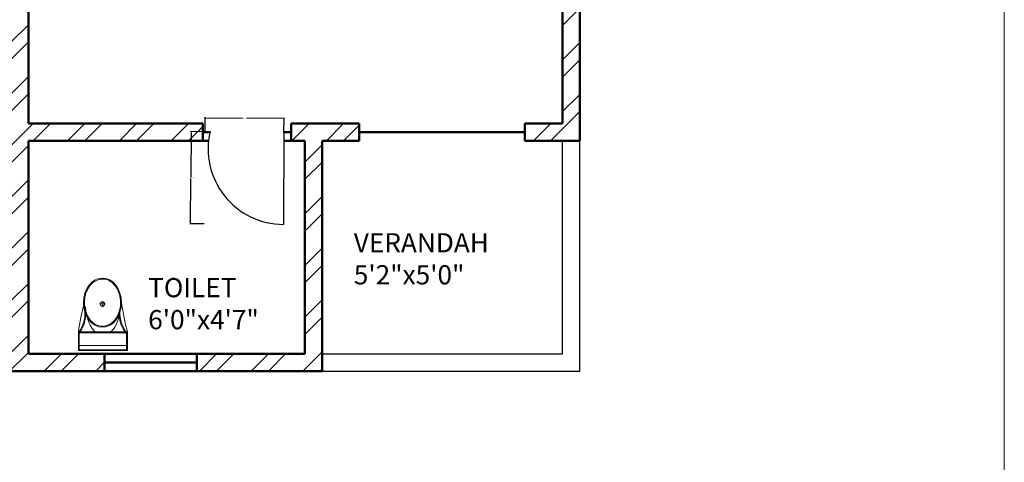
# Model space of a CAD drawing. Units: inches. Extents: x 1901 to 2863, y 888 to 2433.
# Tile 33 of 91: x 2607 to 2863, y 1175 to 1291. Entities that reach past the tile are written whole.
import ezdxf

# ---------------------------------------------------------------- set-up
doc = ezdxf.new("R2010")
doc.units = ezdxf.units.IN
for name, color, linetype, lineweight in [('A-ANNO-DIMS', 2, 'Continuous', 18), ('A-AREA-IDEN', 7, 'Continuous', 18), ('A-DOOR', 4, 'Continuous', 25), ('A-FLOR-FIXT', 9, 'Continuous', 18), ('A-FLOR-HRAL', 41, 'Continuous', 25), ('A-WALL', 7, 'Continuous', 50), ('A-WALL-PATT', 8, 'Continuous', 13)]:
    doc.layers.add(name, color=color, linetype=linetype, lineweight=lineweight)
doc.styles.get("Standard").update_dxf_attribs({"font": 'arial.ttf'})
doc.dimstyles.get("Standard").update_dxf_attribs({"dimtxt": 0.18, "dimasz": 0.18, "dimexe": 0.18, "dimexo": 0.0625, "dimgap": 0.09, "dimtad": 0, "dimtih": 1, "dimtoh": 1, "dimdec": 4, "dimzin": 0, "dimdsep": 46, "dimtxsty": 'Standard', "dimcen": 0.09, "dimadec": 0, "dimazin": 0, "dimtfac": 1, "dimtdec": 4, "dimtofl": 0, "dimtmove": 0, "dimatfit": 3, "dimfxl": 1, "dimtolj": 1, "dimtzin": 0, "dimarcsym": 0})

# ---------------------------------------------------------------- blocks, each defined once
blk = doc.blocks.new('A$C31115884')
for p, q in [((258, 466), (258, 523)), ((283, 498), (223, 498)), ((0, 200), (0, 0)), ((520, 200), (0, 200)), ((10, 190), (10, 10)), ((510, 190), (10, 190)), ((510, 10), (510, 190)), ((520, 0), (520, 200)), ((510, 54), (0, 54)), ((10, 10), (510, 10)), ((0, 0), (520, 0))]:
    blk.add_line(p, q)
blk.add_circle((256, 496), 23.6)
for centre, radius, start, end in [((2778, -205), 2807, 165.4549, 171.7133), ((-295, 403), 365, 324.2091, 9.3499), ((-295, 403), 375, 324.2091, 9.3499), ((139, 406), 293, 315.8436, 2.6563), ((806, 403), 365, 170.6501, 215.7909), ((3237, 905), 2807, 188.2867, 194.5451), ((384, 406), 293, 190.2774, 224.1564), ((806, 403), 375, 179.2036, 215.7909)]:
    blk.add_arc(centre, radius, start, end)
blk.add_ellipse((256, 510), major_axis=(0, -261), ratio=0.772727)
blk.add_open_spline([(256, 259), (263, 259), (270, 260), (288, 262), (299, 265), (320, 273), (330, 278), (350, 291), (360, 299), (378, 316), (386, 326), (402, 347), (409, 358), (421, 383), (427, 395), (436, 422), (440, 436), (445, 465), (447, 480), (448, 509), (448, 524), (445, 553), (443, 568), (436, 596), (432, 610), (422, 636), (416, 649), (402, 672), (395, 683), (379, 703), (370, 712), (351, 728), (341, 735), (321, 746), (310, 751), (289, 757), (278, 759), (256, 761), (245, 761), (223, 757), (212, 754), (191, 746), (181, 741), (161, 728), (151, 720), (133, 703), (125, 693), (110, 672), (103, 660), (90, 636), (85, 623), (76, 596), (72, 582), (67, 553), (66, 538), (64, 509), (65, 494), (68, 465), (70, 450), (77, 422), (81, 408), (91, 382), (97, 370), (111, 346), (118, 335), (135, 316), (144, 307), (162, 291), (172, 284), (193, 273), (203, 269), (225, 262), (236, 260), (250, 259), (253, 259), (256, 259)], degree=3, knots=[0, 0, 0, 0, 0.110105, 0.110105, 0.285049, 0.285049, 0.459994, 0.459994, 0.634938, 0.634938, 0.809882, 0.809882, 0.984827, 0.984827, 1.159771, 1.159771, 1.334715, 1.334715, 1.50966, 1.50966, 1.684604, 1.684604, 1.859549, 1.859549, 2.034493, 2.034493, 2.209437, 2.209437, 2.384382, 2.384382, 2.559326, 2.559326, 2.73427, 2.73427, 2.909215, 2.909215, 3.084159, 3.084159, 3.259103, 3.259103, 3.434048, 3.434048, 3.608992, 3.608992, 3.783936, 3.783936, 3.958881, 3.958881, 4.133825, 4.133825, 4.30877, 4.30877, 4.483714, 4.483714, 4.658658, 4.658658, 4.833603, 4.833603, 5.008547, 5.008547, 5.183491, 5.183491, 5.358436, 5.358436, 5.53338, 5.53338, 5.708324, 5.708324, 5.883269, 5.883269, 6.058213, 6.058213, 6.233158, 6.233158, 6.283185, 6.283185, 6.283185, 6.283185])
blk = doc.blocks.new('DOOR-20')
blk.add_line((0, -0.02), (0, 23.98))
blk.add_arc((0, 4.28), 19.71, 347.419, 90)
blk = doc.blocks.new('*D37')
at = {"layer": 'A-ANNO-DIMS', "color": 0, "lineweight": -2, "transparency": 16777216}
for p, q in [((2655.34, 1261.46), (2651.63, 1261.48)), ((2651.81, 1261.3), (2651.73, 1249.66)), ((2651.66, 1237.66), (2651.73, 1249.3)), ((2655.19, 1237.46), (2651.48, 1237.48))]:
    blk.add_line(p, q, dxfattribs=at)
at = {"layer": 'A-ANNO-DIMS', "color": 0, "transparency": 16777216}
for points in [[(2651.78, 1261.3), (2651.84, 1261.3), (2651.81, 1261.48)], [(2651.63, 1237.66), (2651.69, 1237.66), (2651.66, 1237.48)]]:
    blk.add_solid(points, dxfattribs=at)
at = {"layer": 'Defpoints', "color": 0, "transparency": 16777216}
for p in [(2655.41, 1261.46), (2651.66, 1237.48), (2655.26, 1237.46)]:
    blk.add_point(p, dxfattribs=at)
at = {"layer": 'A-ANNO-DIMS', "color": 0, "transparency": 16777216, "insert": (2651.73, 1249.48), "char_height": 0.18, "attachment_point": 5}
blk.add_mtext('\\A1;DOOR D4 24 TYP.', dxfattribs=at)
blk = doc.blocks.new('*D38')
at = {"layer": 'A-ANNO-DIMS', "color": 0, "lineweight": -2, "transparency": 16777216}
for p, q in [((2655.41, 1261.52), (2655.43, 1265.24)), ((2655.61, 1265.06), (2665.17, 1265)), ((2675.79, 1264.93), (2666.23, 1264.99)), ((2675.94, 1261.39), (2675.97, 1265.11))]:
    blk.add_line(p, q, dxfattribs=at)
at = {"layer": 'A-ANNO-DIMS', "color": 0, "transparency": 16777216}
for points in [[(2655.61, 1265.09), (2655.61, 1265.03), (2655.43, 1265.06)], [(2675.79, 1264.96), (2675.79, 1264.9), (2675.97, 1264.93)]]:
    blk.add_solid(points, dxfattribs=at)
at = {"layer": 'Defpoints', "color": 0, "transparency": 16777216}
for p in [(2655.43, 1265.06), (2655.41, 1261.46), (2675.94, 1261.33)]:
    blk.add_point(p, dxfattribs=at)
at = {"layer": 'A-ANNO-DIMS', "color": 0, "transparency": 16777216, "insert": (2665.7, 1264.99), "char_height": 0.18, "attachment_point": 5}
blk.add_mtext('\\A1;21 TYP.', dxfattribs=at)

msp = doc.modelspace()

# ---------------------------------------------------------------- hatches: boundary and pattern name
at = {"layer": 'A-WALL-PATT'}
h = msp.add_hatch(dxfattribs=at)
h.set_pattern_fill('ANSI32', color=256)
h.paths.add_polyline_path([(2192.5, 2274.13), (2141.26, 2274.13), (2141.26, 2269.63), (2192.5, 2269.63)])
h.paths.add_polyline_path([(2259.93, 2274.13), (2216.5, 2274.13), (2216.5, 2269.63), (2255.43, 2269.63), (2255.43, 2214.63), (2250.81, 2214.63), (2250.81, 2210.13), (2259.93, 2210.13), (2259.93, 2215.13), (2271.76, 2215.13), (2271.76, 2217.38), (2271.76, 2219.63), (2259.93, 2219.63)])
h.paths.add_polyline_path([(2171.43, 2269.63), (2166.93, 2269.63), (2166.93, 2219.63), (2121.24, 2219.63), (2121.24, 2215.13), (2166.93, 2215.13), (2166.93, 2083.13), (2161.81, 2083.13), (2161.81, 2078.63), (2171.43, 2078.63), (2177, 2078.63), (2177, 2080.88), (2177, 2083.13), (2171.43, 2083.13), (2171.43, 2210.13), (2230.91, 2210.13), (2230.91, 2212.38), (2230.91, 2214.63), (2171.43, 2214.63)])
h.paths.add_polyline_path([(2117.26, 2274.13), (2089.43, 2274.13), (2089.43, 2219.63), (2081.14, 2219.63), (2081.14, 2215.13), (2089.43, 2215.13), (2098, 2215.13), (2098, 2217.38), (2098, 2219.63), (2093.93, 2219.63), (2093.93, 2269.63), (2117.26, 2269.63), (2117.26, 2271.88)])
h.paths.add_polyline_path([(2343.43, 2219.63), (2329.29, 2219.63), (2329.29, 2215.13), (2338.93, 2215.13), (2338.93, 2184.74), (2343.43, 2184.74)])
h.paths.add_polyline_path([(2338.93, 2083.13), (2329.29, 2083.13), (2208.97, 2083.13), (2208.97, 2078.63), (2338.93, 2078.63)])
h.paths.add_polyline_path([(2343.43, 2136.74), (2338.93, 2136.74), (2338.93, 1872.63), (2343.43, 1872.63)])
h.paths.add_polyline_path([(2343.43, 1863.63), (2397.68, 1863.63), (2397.68, 1821.63), (2384.14, 1821.63), (2384.14, 1812.63), (2418.33, 1812.63), (2418.33, 1817.13), (2418.33, 1821.63), (2406.68, 1821.63), (2406.68, 1863.63), (2459.5, 1863.63), (2459.5, 1821.63), (2447.14, 1821.63), (2447.14, 1812.63), (2459.5, 1812.63), (2468.5, 1812.63), (2468.5, 1872.63), (2394.43, 1872.63), (2334.43, 1872.63), (2334.43, 1812.63), (2343.43, 1812.63), (2353.25, 1812.63), (2353.25, 1821.63), (2343.43, 1821.63)])
h.paths.add_polyline_path([(2510.01, 1872.63), (2468.5, 1872.63), (2468.5, 1868.13), (2510.01, 1868.13)])
h.paths.add_polyline_path([(2514.01, 1817.13), (2468.5, 1817.13), (2468.5, 1812.63), (2482.11, 1812.63), (2482.11, 1800.61), (2486.61, 1800.61), (2486.61, 1812.63), (2514.01, 1812.63)])
h.paths.add_polyline_path([(2299.25, 1814.88), (2299.25, 1817.13), (2295.93, 1817.13), (2295.93, 1854.17), (2293.68, 1854.17), (2291.43, 1854.17), (2291.43, 1817.13), (2266.11, 1817.13), (2266.11, 1812.63), (2299.25, 1812.63)])
h.paths.add_polyline_path([(2218.11, 1817.13), (2206.46, 1817.13), (2171.43, 1817.13), (2171.43, 1949.13), (2190.1, 1949.13), (2190.1, 1953.63), (2163.47, 1953.63), (2163.47, 1949.13), (2166.93, 1949.13), (2166.93, 1817.13), (2114.3, 1817.13), (2114.3, 1812.63), (2218.11, 1812.63)])
h.paths.add_polyline_path([(2029.43, 1970.92), (2024.93, 1970.92), (2024.93, 1912.72), (2029.43, 1912.72)])
h.paths.add_polyline_path([(2132.3, 1953.63), (2113.93, 1953.63), (2113.93, 1975.89), (2111.68, 1975.89), (2109.43, 1975.89), (2109.43, 1953.63), (2029.43, 1953.63), (2029.43, 1949.13), (2132.3, 1949.13)])
h.paths.add_polyline_path([(2029.43, 1853.61), (2029.31, 1853.61), (2029.31, 1853.61), (2029.43, 1853.61), (2029.43, 1864.72), (2024.93, 1864.72), (2024.93, 1812.63), (2066.3, 1812.63), (2066.3, 1814.88), (2066.3, 1817.13), (2029.43, 1817.13)])
h.paths.add_polyline_path([(2122.93, 2010.09), (2120.68, 2010.09), (2118.43, 2010.09), (2118.43, 2006.13), (2029.43, 2006.13), (2029.43, 2001.63), (2109.43, 2001.63), (2109.43, 1998.04), (2113.93, 1998.04), (2113.93, 2001.63), (2122.93, 2001.63)])
h.paths.add_polyline_path([(2029.43, 2031.38), (2024.93, 2031.38), (2024.93, 1994.92), (2027.18, 1994.92), (2029.43, 1994.92)])
h.paths.add_polyline_path([(2029.43, 2136.74), (2024.93, 2136.74), (2024.93, 2067.38), (2027.18, 2067.38), (2029.43, 2067.38)])
h.paths.add_polyline_path([(2125.62, 2083.13), (2029.43, 2083.13), (2029.43, 2078.63), (2118.43, 2078.63), (2118.43, 2030.71), (2122.93, 2030.71), (2122.93, 2078.63), (2125.62, 2078.63)])
h.paths.add_polyline_path([(2029.43, 2215.13), (2040.47, 2215.13), (2040.47, 2217.38), (2040.47, 2219.63), (2024.93, 2219.63), (2024.93, 2184.74), (2029.43, 2184.74), (2029.43, 2187.78)])
h.paths.add_polyline_path([(2686.43, 2274.13), (2659.28, 2274.13), (2659.28, 2269.63), (2681.93, 2269.63), (2681.93, 2219.63), (2676.82, 2219.63), (2676.82, 2215.13), (2681.93, 2215.13), (2697.01, 2215.13), (2697.01, 2217.38), (2697.01, 2219.63), (2686.43, 2219.63)])
h.paths.add_polyline_path([(2609.93, 2269.63), (2635.28, 2269.63), (2635.28, 2274.13), (2571.43, 2274.13), (2571.43, 2269.63), (2605.43, 2269.63), (2605.43, 2214.63), (2549.1, 2214.63), (2549.1, 2210.13), (2605.43, 2210.13), (2605.43, 2083.13), (2601.01, 2083.13), (2601.01, 2080.88), (2601.01, 2078.63), (2609.93, 2078.63), (2616.16, 2078.63), (2616.16, 2080.88), (2616.16, 2083.13), (2609.93, 2083.13), (2609.93, 2215.13), (2651.46, 2215.13), (2651.46, 2217.38), (2651.46, 2219.63), (2609.93, 2219.63)])
h.paths.add_polyline_path([(2521.43, 2269.63), (2547.43, 2269.63), (2547.43, 2271.88), (2547.43, 2274.13), (2516.93, 2274.13), (2516.93, 2219.63), (2506.41, 2219.63), (2506.41, 2215.13), (2516.93, 2215.13), (2516.93, 2210.13), (2525.4, 2210.13), (2525.4, 2212.38), (2525.4, 2214.63), (2521.43, 2214.63)])
h.paths.add_polyline_path([(2456.01, 2219.63), (2439.43, 2219.63), (2439.43, 2187.89), (2443.93, 2187.89), (2443.93, 2215.13), (2456.01, 2215.13)])
h.paths.add_polyline_path([(2752.93, 2219.63), (2739.48, 2219.63), (2739.48, 2215.13), (2748.43, 2215.13), (2748.43, 2187.89), (2752.93, 2187.89)])
h.paths.add_polyline_path([(2752.93, 2139.89), (2748.43, 2139.89), (2748.43, 2083.13), (2648.42, 2083.13), (2648.42, 2078.63), (2654.93, 2078.63), (2654.93, 2039.44), (2659.43, 2039.44), (2659.43, 2078.63), (2748.43, 2078.63), (2748.43, 2063.43), (2752.93, 2063.43)])
h.paths.add_polyline_path([(2752.93, 2010.63), (2659.43, 2010.63), (2659.43, 2015.65), (2654.93, 2015.65), (2654.93, 2010.63), (2605.43, 2010.63), (2605.43, 1920.97), (2609.93, 1920.97), (2609.93, 2006.13), (2748.43, 2006.13), (2748.43, 1982.47), (2752.93, 1982.47)])
h.paths.add_polyline_path([(2752.93, 2027.43), (2748.43, 2027.43), (2748.43, 2010.63), (2752.93, 2010.63)])
h.paths.add_polyline_path([(2748.43, 1886.13), (2609.93, 1886.13), (2609.93, 1889.72), (2605.43, 1889.72), (2605.43, 1861.26), (2609.93, 1861.26), (2609.93, 1881.63), (2748.43, 1881.63)])
h.paths.add_polyline_path([(2456.86, 2228.83), (2498.4, 2228.83), (2498.4, 2247.49), (2456.86, 2247.49)], flags=9)
h.paths.add_polyline_path([(2038.6, 2237.42), (2080.17, 2237.42), (2080.17, 2256.08), (2038.6, 2256.08)], flags=9)
h.paths.add_polyline_path([(2292.01, 1062.39), (2539.93, 1062.39), (2539.93, 1099.49), (2292.01, 1099.49)], flags=9)
h.paths.add_polyline_path([(2424.91, 1832.25), (2448.51, 1832.25), (2448.51, 1846.68), (2424.91, 1846.68)], flags=25)
h.paths.add_polyline_path([(2359.08, 1832.25), (2382.68, 1832.25), (2382.68, 1846.68), (2359.08, 1846.68)], flags=25)
h.paths.add_polyline_path([(2352.9, 1684.8), (2367.54, 1684.8), (2367.54, 1697.17), (2352.9, 1697.17)], flags=9)
h.paths.add_polyline_path([(2079.29, 1755.83), (2169.02, 1755.83), (2169.02, 1774.37), (2079.29, 1774.37)], flags=9)
h.paths.add_polyline_path([(2404.09, 1373.86), (2404.09, 1463.59), (2385.54, 1463.59), (2385.54, 1373.86)], flags=9)
h.paths.add_polyline_path([(2268.09, 2236.37), (2309.64, 2236.37), (2309.64, 2255.03), (2268.09, 2255.03)], flags=9)
h.paths.add_polyline_path([(2575.96, 1700.95), (2665.7, 1700.95), (2665.7, 1719.5), (2575.96, 1719.5)], flags=9)
h.paths.add_polyline_path([(2302.96, 1878.47), (2329.52, 1878.47), (2329.52, 1888.78), (2302.96, 1888.78)], flags=9)
h.paths.add_polyline_path([(2097.42, 2240.58), (2126.57, 2240.58), (2126.57, 2259.23), (2097.42, 2259.23)], flags=9)
h.paths.add_polyline_path([(2208.72, 2246.12), (2237.88, 2246.12), (2237.88, 2264.78), (2208.72, 2264.78)], flags=9)
h.paths.add_polyline_path([(2038.15, 1925.96), (2076.99, 1925.96), (2076.99, 1944.62), (2038.15, 1944.62)], flags=9)
h.paths.add_polyline_path([(2239.14, 1926.67), (2288.46, 1926.67), (2288.46, 1945.33), (2239.14, 1945.33)], flags=9)
h.paths.add_polyline_path([(2175.43, 2007.33), (2212.36, 2007.33), (2212.36, 2025.99), (2175.43, 2025.99)], flags=9)
h.paths.add_polyline_path([(2225.03, 2091.79), (2263.87, 2091.79), (2263.87, 2110.45), (2225.03, 2110.45)], flags=9)
h.paths.add_polyline_path([(2035.4, 2098.48), (2074.24, 2098.48), (2074.24, 2117.14), (2035.4, 2117.14)], flags=9)
h.paths.add_polyline_path([(2050.1, 2029.21), (2083.26, 2029.21), (2083.26, 2047.87), (2050.1, 2047.87)], flags=9)
h.paths.add_polyline_path([(2069.68, 1956.72), (2098.83, 1956.72), (2098.83, 1975.38), (2069.68, 1975.38)], flags=25)
h.paths.add_polyline_path([(2328.62, 1753.34), (2361.66, 1753.34), (2361.66, 1771.99), (2328.62, 1771.99)], flags=9)
h.paths.add_polyline_path([(2395.16, 2060.89), (2395.16, 2140.65), (2378.68, 2140.65), (2378.68, 2060.89)], flags=9)
h.paths.add_polyline_path([(2463.73, 2059.02), (2492.89, 2059.02), (2492.89, 2077.68), (2463.73, 2077.68)], flags=9)
h.paths.add_polyline_path([(2458.03, 2181.54), (2496.87, 2181.54), (2496.87, 2200.19), (2458.03, 2200.19)], flags=9)
h.paths.add_polyline_path([(2527.58, 2243.07), (2556.73, 2243.07), (2556.73, 2261.73), (2527.58, 2261.73)], flags=9)
h.paths.add_polyline_path([(2694.46, 2232.77), (2736.03, 2232.77), (2736.03, 2251.42), (2694.46, 2251.42)], flags=9)
h.paths.add_polyline_path([(2637.82, 2249.22), (2666.98, 2249.22), (2666.98, 2267.88), (2637.82, 2267.88)], flags=9)
h.paths.add_polyline_path([(2623.69, 2183.54), (2662.53, 2183.54), (2662.53, 2202.2), (2623.69, 2202.2)], flags=9)
h.paths.add_polyline_path([(2691.97, 2021.5), (2725.12, 2021.5), (2725.12, 2040.16), (2691.97, 2040.16)], flags=9)
h.paths.add_polyline_path([(2621.04, 1975.91), (2662.34, 1975.91), (2662.34, 1994.57), (2621.04, 1994.57)], flags=25)
h.paths.add_polyline_path([(2479.03, 1927.62), (2519.84, 1927.62), (2519.84, 1946.28), (2479.03, 1946.28)], flags=9)
h.paths.add_polyline_path([(2670.94, 1849.08), (2716.01, 1849.08), (2716.01, 1867.73), (2670.94, 1867.73)], flags=9)
h.paths.add_polyline_path([(2523.61, 1782.96), (2550.17, 1782.96), (2550.17, 1793.26), (2523.61, 1793.26)], flags=9)
h.paths.add_polyline_path([(2450.84, 1207.33), (2492.39, 1207.33), (2492.39, 1225.99), (2450.84, 1225.99)], flags=9)
h.paths.add_polyline_path([(2527.75, 1203.84), (2556.91, 1203.84), (2556.91, 1222.5), (2527.75, 1222.5)], flags=9)
h.paths.add_polyline_path([(2639.11, 1207.2), (2668.27, 1207.2), (2668.27, 1225.86), (2639.11, 1225.86)], flags=9)
h.paths.add_polyline_path([(2692.59, 1218.97), (2734.17, 1218.97), (2734.17, 1237.62), (2692.59, 1237.62)], flags=9)
h.paths.add_polyline_path([(2669.27, 1366.33), (2708.11, 1366.33), (2708.11, 1384.99), (2669.27, 1384.99)], flags=9)
h.paths.add_polyline_path([(2463.31, 1358.03), (2502.15, 1358.03), (2502.15, 1376.69), (2463.31, 1376.69)], flags=9)
h.paths.add_polyline_path([(2494.72, 1449.96), (2531.65, 1449.96), (2531.65, 1468.62), (2494.72, 1468.62)], flags=9)
h.paths.add_polyline_path([(2675.57, 1422.16), (2708.72, 1422.16), (2708.72, 1440.81), (2675.57, 1440.81)], flags=9)
h.paths.add_polyline_path([(2685.63, 1493.89), (2714.79, 1493.89), (2714.79, 1512.55), (2685.63, 1512.55)], flags=9)
h.paths.add_polyline_path([(2686.8, 1529.91), (2725.65, 1529.91), (2725.65, 1548.57), (2686.8, 1548.57)], flags=9)
h.paths.add_polyline_path([(2503.65, 1537.99), (2552.97, 1537.99), (2552.97, 1556.65), (2503.65, 1556.65)], flags=9)
h.paths.add_polyline_path([(2291.71, 1643.5), (2318.28, 1643.5), (2318.28, 1653.81), (2291.71, 1653.81)], flags=9)
h.paths.add_polyline_path([(2450.63, 1610.52), (2477.19, 1610.52), (2477.19, 1620.82), (2450.63, 1620.82)], flags=9)
h.paths.add_polyline_path([(2359.99, 1551.81), (2422.25, 1551.81), (2422.25, 1562.12), (2359.99, 1562.12)], flags=9)
h.paths.add_polyline_path([(2280.11, 1249.01), (2321.65, 1249.01), (2321.65, 1267.66), (2280.11, 1267.66)], flags=9)
h.paths.add_polyline_path([(2164.06, 1274.23), (2193.22, 1274.23), (2193.22, 1292.89), (2164.06, 1292.89)], flags=9)
h.paths.add_polyline_path([(2118.21, 1277.69), (2151.25, 1277.69), (2151.25, 1296.35), (2118.21, 1296.35)], flags=9)
h.paths.add_polyline_path([(2031.95, 1268.53), (2073.52, 1268.53), (2073.52, 1287.19), (2031.95, 1287.19)], flags=9)
h.paths.add_polyline_path([(2050.2, 1409.08), (2089.04, 1409.08), (2089.04, 1427.74), (2050.2, 1427.74)], flags=9)
h.paths.add_polyline_path([(2243.74, 1421.03), (2282.58, 1421.03), (2282.58, 1439.69), (2243.74, 1439.69)], flags=9)
h.paths.add_polyline_path([(2190.75, 1509.77), (2231.56, 1509.77), (2231.56, 1528.43), (2190.75, 1528.43)], flags=9)
h.paths.add_polyline_path([(2058.39, 1475.42), (2091.55, 1475.42), (2091.55, 1494.07), (2058.39, 1494.07)], flags=9)
h.paths.add_polyline_path([(2062.45, 1553.09), (2091.6, 1553.09), (2091.6, 1571.75), (2062.45, 1571.75)], flags=9)
h.paths.add_polyline_path([(2219.52, 1590.37), (2266.15, 1590.37), (2266.15, 1609.02), (2219.52, 1609.02)], flags=9)
h.paths.add_polyline_path([(2041.07, 1584.19), (2079.91, 1584.19), (2079.91, 1602.85), (2041.07, 1602.85)], flags=9)
h = msp.add_hatch(dxfattribs=at)
h.set_pattern_fill('ANSI32', color=256)
h.paths.add_polyline_path([(2443.93, 2139.89), (2439.43, 2139.89), (2439.43, 2069.35), (2441.68, 2069.35), (2443.93, 2069.35), (2443.93, 2078.63), (2521.93, 2078.63), (2521.93, 2075.07), (2524.18, 2075.07), (2526.43, 2075.07), (2526.43, 2078.63), (2571.75, 2078.63), (2571.75, 2080.88), (2571.75, 2083.13), (2443.93, 2083.13)])
h.paths.add_polyline_path([(2526.43, 2054.63), (2524.18, 2054.63), (2521.93, 2054.63), (2521.93, 2030.63), (2443.93, 2030.63), (2443.93, 2045.35), (2439.43, 2045.35), (2439.43, 1983.87), (2443.93, 1983.87), (2443.93, 2026.13), (2521.93, 2026.13), (2526.43, 2026.13)])
h.paths.add_polyline_path([(2443.93, 1923.87), (2439.43, 1923.87), (2439.43, 1872.63), (2443.93, 1872.63)])
h.paths.add_polyline_path([(2636.23, 1766.13), (2609.93, 1766.13), (2609.93, 1779.79), (2605.43, 1779.79), (2605.43, 1766.13), (2486.61, 1766.13), (2486.61, 1770.67), (2482.11, 1770.67), (2482.11, 1766.13), (2482.11, 1761.63), (2636.23, 1761.63), (2636.23, 1763.88)])
h.paths.add_polyline_path([(2519.54, 1663.38), (2519.54, 1665.63), (2494.93, 1665.63), (2481.83, 1665.63), (2481.83, 1663.38), (2481.83, 1661.13), (2490.43, 1661.13), (2490.43, 1640.16), (2494.93, 1640.16), (2494.93, 1661.13), (2519.54, 1661.13)])
h.paths.add_polyline_path([(2443.93, 1712.13), (2443.93, 1716.63), (2414.46, 1716.63), (2414.46, 1712.13), (2439.43, 1712.13), (2439.43, 1545.51), (2443.93, 1545.51), (2443.93, 1661.13), (2448.47, 1661.13), (2448.47, 1665.63), (2443.93, 1665.63)])
h.paths.add_polyline_path([(2343.43, 1712.13), (2365.52, 1712.13), (2365.52, 1714.38), (2365.52, 1716.63), (2333.87, 1716.63), (2333.87, 1714.38), (2333.87, 1712.13), (2338.93, 1712.13), (2338.93, 1575.63), (2338.93, 1545.51), (2343.43, 1545.51), (2343.43, 1547.51), (2343.43, 1580.13)])
h.paths.add_polyline_path([(2752.93, 1665.63), (2579.54, 1665.63), (2579.54, 1661.13), (2615.93, 1661.13), (2615.93, 1529.13), (2598.93, 1529.13), (2598.93, 1524.63), (2623.13, 1524.63), (2623.13, 1526.88), (2623.13, 1529.13), (2620.43, 1529.13), (2620.43, 1661.13), (2748.43, 1661.13), (2748.43, 1633.5), (2752.93, 1633.5)])
h.paths.add_polyline_path([(2752.93, 1419.93), (2748.43, 1419.93), (2748.43, 1400.13), (2659.43, 1400.13), (2659.43, 1444.33), (2657.18, 1444.33), (2654.93, 1444.33), (2654.93, 1400.13), (2643.65, 1400.13), (2643.65, 1395.63), (2748.43, 1395.63), (2748.43, 1364.04), (2752.93, 1364.04)])
h.paths.add_polyline_path([(2752.93, 1492.88), (2748.43, 1492.88), (2748.43, 1476.63), (2667.43, 1476.63), (2667.43, 1479.71), (2665.18, 1479.71), (2662.93, 1479.71), (2662.93, 1476.63), (2654.93, 1476.63), (2654.93, 1469.54), (2659.43, 1469.54), (2659.43, 1472.13), (2748.43, 1472.13), (2748.43, 1455.93), (2752.93, 1455.93)])
h.paths.add_polyline_path([(2752.93, 1304.04), (2748.43, 1304.04), (2748.43, 1263.63), (2738.66, 1263.63), (2738.66, 1259.13), (2752.93, 1259.13)])
h.paths.add_polyline_path([(2685.93, 1259.13), (2695.49, 1259.13), (2695.49, 1261.38), (2695.49, 1263.63), (2677.84, 1263.63), (2677.84, 1261.38), (2677.84, 1259.13), (2681.43, 1259.13), (2681.43, 1203.63), (2653.28, 1203.63), (2653.28, 1199.13), (2685.93, 1199.13), (2685.93, 1203.63)])
h.paths.add_polyline_path([(2609.43, 1395.63), (2611.85, 1395.63), (2611.85, 1400.13), (2598.89, 1400.13), (2598.89, 1397.88), (2598.89, 1395.63), (2604.93, 1395.63), (2604.93, 1268.13), (2554.73, 1268.13), (2554.73, 1265.88), (2554.73, 1263.63), (2604.93, 1263.63), (2604.93, 1203.63), (2571.31, 1203.63), (2571.31, 1199.13), (2604.93, 1199.13), (2629.28, 1199.13), (2629.28, 1201.38), (2629.28, 1203.63), (2609.43, 1203.63), (2609.43, 1258.63), (2609.43, 1259.13), (2654.8, 1259.13), (2654.8, 1263.63), (2609.43, 1263.63)])
h.paths.add_polyline_path([(2443.93, 1304.04), (2439.43, 1304.04), (2439.43, 1259.13), (2443.93, 1259.13), (2456.16, 1259.13), (2456.16, 1261.38), (2456.16, 1263.63), (2443.93, 1263.63)])
h.paths.add_polyline_path([(2525.43, 1263.63), (2531.78, 1263.63), (2531.78, 1268.13), (2520.93, 1268.13), (2520.93, 1263.63), (2511.41, 1263.63), (2511.41, 1259.13), (2520.93, 1259.13), (2520.93, 1199.13), (2547.31, 1199.13), (2547.31, 1201.38), (2547.31, 1203.63), (2525.43, 1203.63)])
h.paths.add_polyline_path([(2443.93, 1434.84), (2439.43, 1434.84), (2439.43, 1364.04), (2441.68, 1364.04), (2443.93, 1364.04)])
h.paths.add_polyline_path([(2567.13, 1400.13), (2443.93, 1400.13), (2443.93, 1395.63), (2567.13, 1395.63)])
h.paths.add_polyline_path([(2443.93, 1545.51), (2439.43, 1545.51), (2439.43, 1494.84), (2443.93, 1494.84)])
h.paths.add_polyline_path([(2494.93, 1553.35), (2492.68, 1553.35), (2490.43, 1553.35), (2490.43, 1524.63), (2494.93, 1524.63), (2525.94, 1524.63), (2525.94, 1526.88), (2525.94, 1529.13), (2494.93, 1529.13)])
h.paths.add_polyline_path([(2752.93, 1573.5), (2748.43, 1573.5), (2748.43, 1529.13), (2657.76, 1529.13), (2657.76, 1524.63), (2662.93, 1524.63), (2662.93, 1498.63), (2667.43, 1498.63), (2667.43, 1524.63), (2748.43, 1524.63), (2748.43, 1516.88), (2752.93, 1516.88)])
h.paths.add_polyline_path([(2038.6, 2237.42), (2080.17, 2237.42), (2080.17, 2256.08), (2038.6, 2256.08)], flags=9)
h.paths.add_polyline_path([(2292.01, 1062.39), (2539.93, 1062.39), (2539.93, 1099.49), (2292.01, 1099.49)], flags=9)
h.paths.add_polyline_path([(2424.91, 1832.25), (2448.51, 1832.25), (2448.51, 1846.68), (2424.91, 1846.68)], flags=9)
h.paths.add_polyline_path([(2359.08, 1832.25), (2382.68, 1832.25), (2382.68, 1846.68), (2359.08, 1846.68)], flags=9)
h.paths.add_polyline_path([(2352.9, 1684.8), (2367.54, 1684.8), (2367.54, 1697.17), (2352.9, 1697.17)], flags=9)
h.paths.add_polyline_path([(2079.29, 1755.83), (2169.02, 1755.83), (2169.02, 1774.37), (2079.29, 1774.37)], flags=9)
h.paths.add_polyline_path([(2404.09, 1373.86), (2404.09, 1463.59), (2385.54, 1463.59), (2385.54, 1373.86)], flags=9)
h.paths.add_polyline_path([(2268.09, 2236.37), (2309.64, 2236.37), (2309.64, 2255.03), (2268.09, 2255.03)], flags=9)
h.paths.add_polyline_path([(2575.96, 1700.95), (2665.7, 1700.95), (2665.7, 1719.5), (2575.96, 1719.5)], flags=9)
h.paths.add_polyline_path([(2302.96, 1878.47), (2329.52, 1878.47), (2329.52, 1888.78), (2302.96, 1888.78)], flags=9)
h.paths.add_polyline_path([(2097.42, 2240.58), (2126.57, 2240.58), (2126.57, 2259.23), (2097.42, 2259.23)], flags=9)
h.paths.add_polyline_path([(2208.72, 2246.12), (2237.88, 2246.12), (2237.88, 2264.78), (2208.72, 2264.78)], flags=9)
h.paths.add_polyline_path([(2038.15, 1925.96), (2076.99, 1925.96), (2076.99, 1944.62), (2038.15, 1944.62)], flags=9)
h.paths.add_polyline_path([(2239.14, 1926.67), (2288.46, 1926.67), (2288.46, 1945.33), (2239.14, 1945.33)], flags=9)
h.paths.add_polyline_path([(2175.43, 2007.33), (2212.36, 2007.33), (2212.36, 2025.99), (2175.43, 2025.99)], flags=9)
h.paths.add_polyline_path([(2225.03, 2091.79), (2263.87, 2091.79), (2263.87, 2110.45), (2225.03, 2110.45)], flags=9)
h.paths.add_polyline_path([(2035.4, 2098.48), (2074.24, 2098.48), (2074.24, 2117.14), (2035.4, 2117.14)], flags=9)
h.paths.add_polyline_path([(2050.1, 2029.21), (2083.26, 2029.21), (2083.26, 2047.87), (2050.1, 2047.87)], flags=9)
h.paths.add_polyline_path([(2069.68, 1956.72), (2098.83, 1956.72), (2098.83, 1975.38), (2069.68, 1975.38)], flags=9)
h.paths.add_polyline_path([(2328.62, 1753.34), (2361.66, 1753.34), (2361.66, 1771.99), (2328.62, 1771.99)], flags=9)
h.paths.add_polyline_path([(2395.16, 2060.89), (2395.16, 2140.65), (2378.68, 2140.65), (2378.68, 2060.89)], flags=9)
h.paths.add_polyline_path([(2463.73, 2059.02), (2492.89, 2059.02), (2492.89, 2077.68), (2463.73, 2077.68)], flags=9)
h.paths.add_polyline_path([(2458.03, 2181.54), (2496.87, 2181.54), (2496.87, 2200.19), (2458.03, 2200.19)], flags=9)
h.paths.add_polyline_path([(2456.86, 2228.83), (2498.4, 2228.83), (2498.4, 2247.49), (2456.86, 2247.49)], flags=9)
h.paths.add_polyline_path([(2527.58, 2243.07), (2556.73, 2243.07), (2556.73, 2261.73), (2527.58, 2261.73)], flags=9)
h.paths.add_polyline_path([(2694.46, 2232.77), (2736.03, 2232.77), (2736.03, 2251.42), (2694.46, 2251.42)], flags=9)
h.paths.add_polyline_path([(2637.82, 2249.22), (2666.98, 2249.22), (2666.98, 2267.88), (2637.82, 2267.88)], flags=9)
h.paths.add_polyline_path([(2623.69, 2183.54), (2662.53, 2183.54), (2662.53, 2202.2), (2623.69, 2202.2)], flags=9)
h.paths.add_polyline_path([(2691.97, 2021.5), (2725.12, 2021.5), (2725.12, 2040.16), (2691.97, 2040.16)], flags=9)
h.paths.add_polyline_path([(2621.04, 1975.91), (2662.34, 1975.91), (2662.34, 1994.57), (2621.04, 1994.57)], flags=9)
h.paths.add_polyline_path([(2479.03, 1927.62), (2519.84, 1927.62), (2519.84, 1946.28), (2479.03, 1946.28)], flags=9)
h.paths.add_polyline_path([(2670.94, 1849.08), (2716.01, 1849.08), (2716.01, 1867.73), (2670.94, 1867.73)], flags=9)
h.paths.add_polyline_path([(2523.61, 1782.96), (2550.17, 1782.96), (2550.17, 1793.26), (2523.61, 1793.26)], flags=9)
h.paths.add_polyline_path([(2450.84, 1207.33), (2492.39, 1207.33), (2492.39, 1225.99), (2450.84, 1225.99)], flags=9)
h.paths.add_polyline_path([(2527.75, 1203.84), (2556.91, 1203.84), (2556.91, 1222.5), (2527.75, 1222.5)], flags=9)
h.paths.add_polyline_path([(2639.11, 1207.2), (2668.27, 1207.2), (2668.27, 1225.86), (2639.11, 1225.86)], flags=9)
h.paths.add_polyline_path([(2692.59, 1218.97), (2734.17, 1218.97), (2734.17, 1237.62), (2692.59, 1237.62)], flags=9)
h.paths.add_polyline_path([(2669.27, 1366.33), (2708.11, 1366.33), (2708.11, 1384.99), (2669.27, 1384.99)], flags=25)
h.paths.add_polyline_path([(2463.31, 1358.03), (2502.15, 1358.03), (2502.15, 1376.69), (2463.31, 1376.69)], flags=9)
h.paths.add_polyline_path([(2494.72, 1449.96), (2531.65, 1449.96), (2531.65, 1468.62), (2494.72, 1468.62)], flags=9)
h.paths.add_polyline_path([(2675.57, 1422.16), (2708.72, 1422.16), (2708.72, 1440.81), (2675.57, 1440.81)], flags=25)
h.paths.add_polyline_path([(2685.63, 1493.89), (2714.79, 1493.89), (2714.79, 1512.55), (2685.63, 1512.55)], flags=9)
h.paths.add_polyline_path([(2686.8, 1529.91), (2725.65, 1529.91), (2725.65, 1548.57), (2686.8, 1548.57)], flags=25)
h.paths.add_polyline_path([(2503.65, 1537.99), (2552.97, 1537.99), (2552.97, 1556.65), (2503.65, 1556.65)], flags=9)
h.paths.add_polyline_path([(2291.71, 1643.5), (2318.28, 1643.5), (2318.28, 1653.81), (2291.71, 1653.81)], flags=9)
h.paths.add_polyline_path([(2450.63, 1610.52), (2477.19, 1610.52), (2477.19, 1620.82), (2450.63, 1620.82)], flags=9)
h.paths.add_polyline_path([(2359.99, 1551.81), (2422.25, 1551.81), (2422.25, 1562.12), (2359.99, 1562.12)], flags=9)
h.paths.add_polyline_path([(2280.11, 1249.01), (2321.65, 1249.01), (2321.65, 1267.66), (2280.11, 1267.66)], flags=9)
h.paths.add_polyline_path([(2164.06, 1274.23), (2193.22, 1274.23), (2193.22, 1292.89), (2164.06, 1292.89)], flags=9)
h.paths.add_polyline_path([(2118.21, 1277.69), (2151.25, 1277.69), (2151.25, 1296.35), (2118.21, 1296.35)], flags=9)
h.paths.add_polyline_path([(2031.95, 1268.53), (2073.52, 1268.53), (2073.52, 1287.19), (2031.95, 1287.19)], flags=9)
h.paths.add_polyline_path([(2050.2, 1409.08), (2089.04, 1409.08), (2089.04, 1427.74), (2050.2, 1427.74)], flags=9)
h.paths.add_polyline_path([(2243.74, 1421.03), (2282.58, 1421.03), (2282.58, 1439.69), (2243.74, 1439.69)], flags=9)
h.paths.add_polyline_path([(2190.75, 1509.77), (2231.56, 1509.77), (2231.56, 1528.43), (2190.75, 1528.43)], flags=9)
h.paths.add_polyline_path([(2058.39, 1475.42), (2091.55, 1475.42), (2091.55, 1494.07), (2058.39, 1494.07)], flags=9)
h.paths.add_polyline_path([(2062.45, 1553.09), (2091.6, 1553.09), (2091.6, 1571.75), (2062.45, 1571.75)], flags=9)
h.paths.add_polyline_path([(2219.52, 1590.37), (2266.15, 1590.37), (2266.15, 1609.02), (2219.52, 1609.02)], flags=9)
h.paths.add_polyline_path([(2041.07, 1584.19), (2079.91, 1584.19), (2079.91, 1602.85), (2041.07, 1602.85)], flags=9)

# ---------------------------------------------------------------- linework, layer by layer
at = {"layer": 'A-FLOR-FIXT'}
msp.add_lwpolyline([(1901.45, 2433.12), (2863.43, 2433.12), (2863.43, 961.82), (1901.45, 961.82)], close=True, dxfattribs=at)
at = {"layer": 'A-FLOR-HRAL'}
for p, q in [((2748.43, 1203.63), (2748.43, 1259.13)), ((2752.93, 1199.13), (2752.93, 1259.13)), ((2685.93, 1203.63), (2748.43, 1203.63)), ((2685.93, 1199.13), (2752.93, 1199.13))]:
    msp.add_line(p, q, dxfattribs=at)
at = {"layer": 'A-WALL'}
for p, q in [((2752.93, 1665.63), (2752.93, 1259.13)), ((2609.43, 1395.63), (2609.43, 1263.63)), ((2748.43, 1395.63), (2748.43, 1263.63)), ((2609.43, 1263.63), (2654.8, 1263.63)), ((2654.8, 1259.13), (2654.8, 1263.63)), ((2654.8, 1263.63), (2654.8, 1261.38)), ((2677.84, 1259.13), (2677.84, 1263.63)), ((2677.84, 1263.63), (2677.84, 1261.38)), ((2677.84, 1263.63), (2695.49, 1263.63)), ((2695.49, 1263.63), (2695.49, 1259.13)), ((2738.66, 1261.38), (2738.66, 1263.63)), ((2738.66, 1263.63), (2738.66, 1259.13)), ((2738.66, 1263.63), (2748.43, 1263.63)), ((2654.8, 1261.38), (2656.8, 1261.38)), ((2677.84, 1261.38), (2675.84, 1261.38)), ((2695.49, 1259.13), (2695.49, 1261.38)), ((2695.49, 1261.38), (2738.66, 1261.38)), ((2609.43, 1259.13), (2609.43, 1203.63)), ((2609.43, 1259.13), (2656.41, 1259.13)), ((2609.43, 1203.63), (2609.43, 1258.63)), ((2675.84, 1259.13), (2681.43, 1259.13)), ((2681.43, 1203.63), (2681.43, 1259.13)), ((2685.93, 1259.13), (2685.93, 1203.63)), ((2685.93, 1259.13), (2695.49, 1259.13)), ((2738.66, 1259.13), (2752.93, 1259.13)), ((2609.43, 1203.63), (2681.43, 1203.63)), ((2629.28, 1203.63), (2629.28, 1199.13)), ((2653.28, 1201.38), (2653.28, 1203.63)), ((2653.28, 1203.63), (2653.28, 1199.13)), ((2685.93, 1203.63), (2685.93, 1199.13)), ((2629.28, 1199.13), (2629.28, 1201.38)), ((2629.28, 1201.38), (2653.28, 1201.38)), ((2685.93, 1199.13), (2604.93, 1199.13)), ((2629.28, 1199.13), (2629.28, 1199.13))]:
    msp.add_line(p, q, dxfattribs=at)

# ---------------------------------------------------------------- block references
at = {"layer": 'A-DOOR', "rotation": 179.6372118038556}
msp.add_blockref('DOOR-20', (2675.95, 1261.31), dxfattribs=at)
at = {"layer": 'A-FLOR-FIXT', "xscale": 0.0245149588751191, "yscale": 0.0245149588751191, "zscale": 0.0245149588751191}
msp.add_blockref('A$C31115884', (2622.45, 1204.46), dxfattribs=at)

# ---------------------------------------------------------------- texts
at = {"layer": 'A-AREA-IDEN', "char_height": 5, "attachment_point": 1}
for s, width, insert in [('VERANDAH\\P5\'2"x5\'0"', 165.1722, (2694.13, 1235.05)), ('TOILET\\P6\'0"x4\'7"', 120.5435, (2640.62, 1223.37))]:
    msp.add_mtext_dynamic_manual_height_columns(s, width=width, gutter_width=12.5, heights=[0], dxfattribs=dict(at, insert=insert))

# ---------------------------------------------------------------- dimensions: what is measured, and where the dimension line sits
at = {"layer": 'A-ANNO-DIMS'}
for base, p1, p2, angle, text, picture, middle in [((2655.43, 1265.06), (2675.94, 1261.33), (2655.41, 1261.46), 179.6372, '<> TYP.', '*D38', (2665.7, 1264.99)), ((2651.66, 1237.48), (2655.41, 1261.46), (2655.26, 1237.46), 269.6372, 'DOOR D4 <> TYP.', '*D37', (2651.73, 1249.48))]:
    dim = msp.add_linear_dim(base=base, p1=p1, p2=p2, angle=angle, text=text, dimstyle='Standard', override={"dimdec": 0, "dimlfac": 1, "dimrnd": 0, "dimzin": 0, "dimdsep": 46, "dimlunit": 2}, dxfattribs=at)
    dim.commit()
    dim.dimension.update_dxf_attribs({"geometry": picture, "text_midpoint": middle})

doc.saveas('drawing.dxf')
